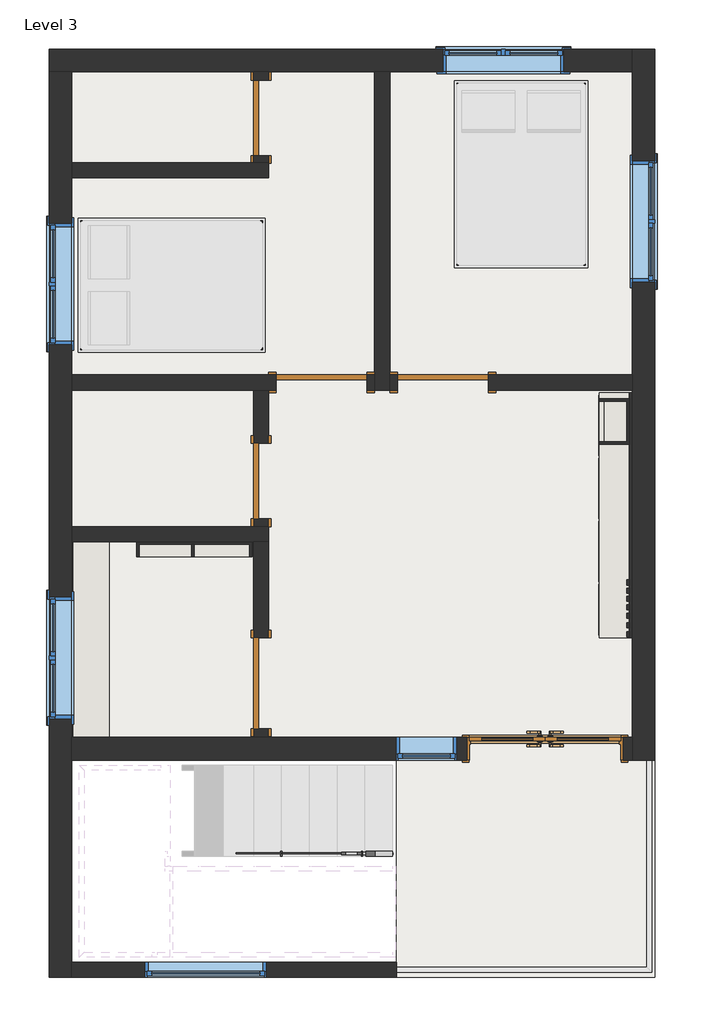
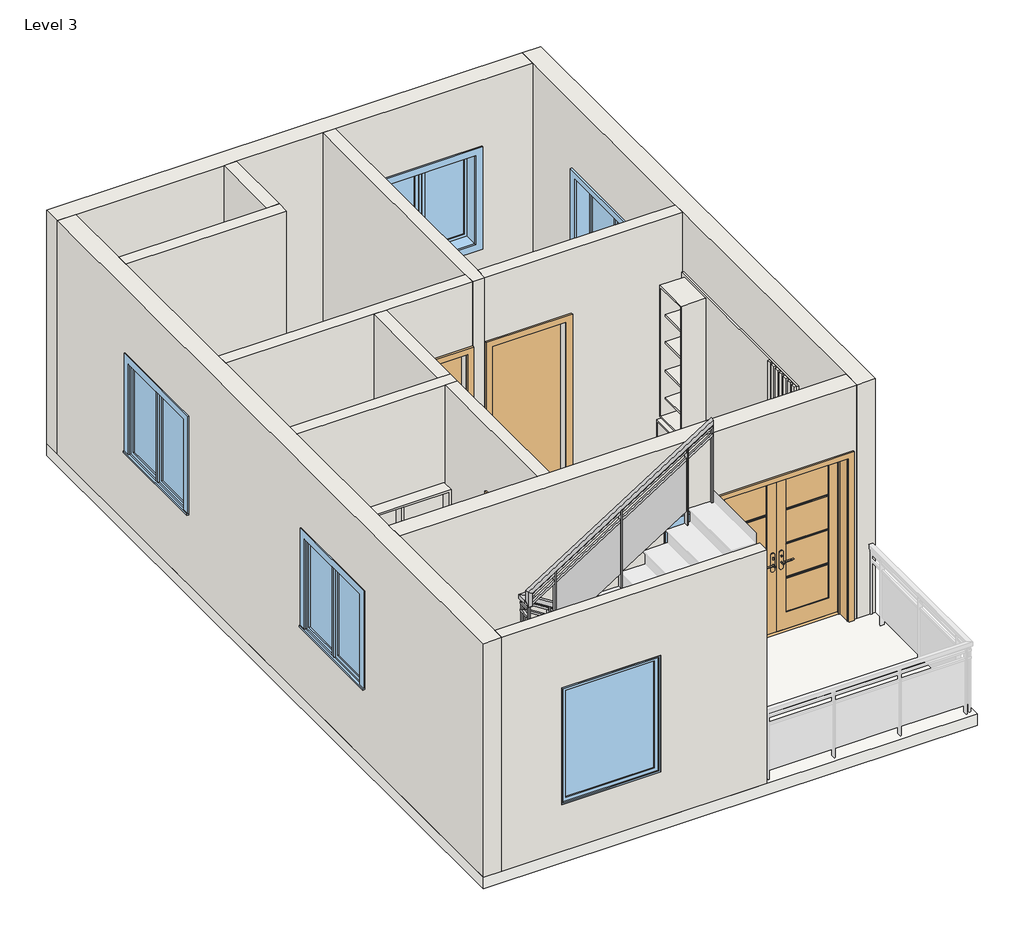
# One storey, part 1 of 2: 15 walls, 6 doors, 6 windows, 1 railing, 1 slab.
"""IFC4 building model written with IfcOpenShell, lengths in millimetres."""

from ifc_helpers import new_model, si_unit, frame, origin, place, context, project, spatial, polyline, outline, extrude, faceted_brep, transform, mapped, element, save
from components import m_door_exterior_double_full_glass_wood_clad_1524_x_2134mm_606f56d5, single_flush_2_5_e2b13fe9, door_686f89d2, door_16372e1c, walls_5_walls_1_1b2d60d9, walls_6_walls_2_a14d7d6d, window_534dcd48, window_fc882ab3, fixed_4_86eadd64

model = new_model("IFC4")

# Units and contexts
model_context = context("Model", 3, world=origin())
ifc_project = project(units=[si_unit("LENGTHUNIT", "METRE", prefix="MILLI")], contexts=[model_context])

# Site, building, storey
site = spatial("IfcSite", under=ifc_project)
building = spatial("IfcBuilding", under=site)
storey = spatial("IfcBuildingStorey", under=building, Name="Level 3", Elevation=6400.8)

# Doors
placement = place(None, origin())
m_door_exterior_double_full_glass_wood_clad_1524_x_2134mm_shape = m_door_exterior_double_full_glass_wood_clad_1524_x_2134mm_606f56d5(model_context)
element("IfcDoor", 1, ObjectType="M_Door-Exterior-Double-Full Glass-Wood_Clad : 1524 x 2134mm", at=placement, inside=storey, context=model_context, shape_type="MappedRepresentation", body=[
    mapped(m_door_exterior_double_full_glass_wood_clad_1524_x_2134mm_shape, transform((-1708.6112714, -4701.782676, 6400.8), x_axis=(1.0, 0.0, 0.0), y_axis=(0.0, 1.0, 0.0), z_axis=(0.0, 0.0, 1.0))),
])
single_flush_2_5_shape = single_flush_2_5_e2b13fe9(model_context)
element("IfcDoor", 2, ObjectType="Single-Flush : 2.5'", at=placement, inside=storey, context=model_context, shape_type="MappedRepresentation", body=[
    mapped(single_flush_2_5_shape, transform((-4566.1112714, -2012.557676, 6400.8), x_axis=(0.0, -1.0, 0.0), y_axis=(1.0, 0.0, 0.0), z_axis=(0.0, 0.0, 1.0))),
])
element("IfcDoor", 3, ObjectType="Single-Flush : 2.5'", at=placement, inside=storey, context=model_context, shape_type="MappedRepresentation", body=[
    mapped(single_flush_2_5_shape, transform((-4566.1112714, 1638.692324, 6400.8), x_axis=(0.0, -1.0, 0.0), y_axis=(1.0, 0.0, 0.0), z_axis=(0.0, 0.0, 1.0))),
])
door_shape = door_686f89d2(model_context)
element("IfcDoor", 4, ObjectType="Single-Flush : 36\" x 84\"", at=placement, inside=storey, context=model_context, shape_type="MappedRepresentation", body=[
    mapped(door_shape, transform((-4566.1112714, -4044.557676, 6400.8), x_axis=(0.0, -1.0, 0.0), y_axis=(1.0, 0.0, 0.0), z_axis=(0.0, 0.0, 1.0))),
])
element("IfcDoor", 5, ObjectType="Single-Flush : 36\" x 84\"", at=placement, inside=storey, context=model_context, shape_type="MappedRepresentation", body=[
    mapped(door_shape, transform((-2737.3112714, -1021.957676, 6400.8), x_axis=(-1.0, 0.0, 0.0), y_axis=(0.0, -1.0, 0.0), z_axis=(0.0, 0.0, 1.0))),
])
door_2_shape = door_16372e1c(model_context)
element("IfcDoor", 6, ObjectType="Single-Flush : 36\" x 84\"", at=placement, inside=storey, context=model_context, shape_type="MappedRepresentation", body=[
    mapped(door_2_shape, transform((-3956.5112714, -1021.957676, 6400.8), x_axis=(1.0, 0.0, 0.0), y_axis=(0.0, 1.0, 0.0), z_axis=(0.0, 0.0, 1.0))),
])

# Railing
element("IfcRailing", 7, ObjectType="Glass Panel - Bottom Fill", at=placement, inside=storey, context=model_context, shape_type="SolidModel", body=[
    faceted_brep([(-5531.3112714, -5886.057676, 9060.8727273), (-5480.5112714, -5886.057676, 9032.986276), (-5480.5112714, -5936.857676, 9032.986276), (-5531.3112714, -5936.857676, 9060.8727273), (-3245.3112714, -5886.057676, 10515.6), (-3245.3112714, -5936.857676, 10515.6), (-3245.3112714, -5936.857676, 10455.386276), (-3245.3112714, -5886.057676, 10455.386276)], [[[0, 1, 2, 3]], [[4, 5, 6, 7]], [[1, 0, 4, 7]], [[2, 1, 7, 6]], [[3, 2, 6, 5]], [[0, 3, 5, 4]]]),
    faceted_brep([(-5480.5112714, -5886.057676, 8915.4), (-5531.3112714, -5886.057676, 8915.4), (-5531.3112714, -5936.857676, 8864.6), (-5480.5112714, -5936.857676, 8864.6), (-5480.5112714, -5860.657676, 8864.6), (-5480.5112714, -5860.657676, 8915.4), (-5531.3112714, -5860.657676, 8864.6), (-5531.3112714, -5860.657676, 8915.4), (-3245.3112714, -5784.457676, 7493.0), (-3245.3112714, -5784.457676, 7432.786276), (-3245.3112714, -5733.657676, 7432.786276), (-3245.3112714, -5733.657676, 7493.0), (-5404.3112714, -5784.457676, 8866.9090909), (-5455.1112714, -5784.457676, 8839.0226396), (-5455.1112714, -5733.657676, 8839.0226396), (-5404.3112714, -5733.657676, 8866.9090909), (-5404.3112714, -5784.457676, 8915.4), (-5455.1112714, -5784.457676, 8864.6), (-5455.1112714, -5733.657676, 8864.6), (-5404.3112714, -5733.657676, 8915.4), (-5480.5112714, -5784.457676, 8915.4), (-5480.5112714, -5784.457676, 8864.6), (-5531.3112714, -5733.657676, 8864.6), (-5531.3112714, -5733.657676, 8915.4)], [[[0, 1, 2, 3]], [[4, 5, 0, 3]], [[6, 4, 3, 2]], [[7, 6, 2, 1]], [[5, 7, 1, 0]], [[8, 9, 10, 11]], [[9, 8, 12, 13]], [[10, 9, 13, 14]], [[11, 10, 14, 15]], [[8, 11, 15, 12]], [[13, 12, 16, 17]], [[14, 13, 17, 18]], [[15, 14, 18, 19]], [[12, 15, 19, 16]], [[17, 16, 20, 21]], [[18, 17, 21, 22]], [[19, 18, 22, 23]], [[16, 19, 23, 20]], [[21, 20, 5, 4]], [[22, 21, 4, 6]], [[23, 22, 6, 7]], [[20, 23, 7, 5]]]),
    faceted_brep([(-5480.5112714, -5886.057676, 8915.4), (-5480.5112714, -5936.857676, 8864.6), (-5531.3112714, -5936.857676, 8864.6), (-5531.3112714, -5886.057676, 8915.4), (-5480.5112714, -5886.057676, 9032.986276), (-5531.3112714, -5886.057676, 9060.8727273), (-5531.3112714, -5936.857676, 9060.8727273), (-5480.5112714, -5936.857676, 9032.986276)], [[[0, 1, 2, 3]], [[4, 5, 6, 7]], [[1, 0, 4, 7]], [[2, 1, 7, 6]], [[3, 2, 6, 5]], [[0, 3, 5, 4]]]),
    faceted_brep([(-3245.3112714, -5771.757676, 7406.453431), (-3245.3112714, -5771.757676, 7376.346569), (-3245.3112714, -5746.357676, 7376.346569), (-3245.3112714, -5746.357676, 7406.453431), (-5476.8130227, -5771.757676, 8826.5), (-5484.2095201, -5771.757676, 8801.1), (-5484.2095201, -5746.357676, 8801.1), (-5476.8130227, -5746.357676, 8826.5), (-5493.2112714, -5771.757676, 8826.5), (-5493.2112714, -5771.757676, 8801.1), (-5518.6112714, -5746.357676, 8801.1), (-5518.6112714, -5746.357676, 8826.5), (-5493.2112714, -5898.757676, 8826.5), (-5518.6112714, -5898.757676, 8826.5), (-5518.6112714, -5898.757676, 8801.1), (-5493.2112714, -5898.757676, 8801.1)], [[[0, 1, 2, 3]], [[1, 0, 4, 5]], [[2, 1, 5, 6]], [[3, 2, 6, 7]], [[0, 3, 7, 4]], [[5, 4, 8, 9]], [[6, 5, 9, 10]], [[7, 6, 10, 11]], [[4, 7, 11, 8]], [[12, 13, 14, 15]], [[9, 8, 12, 15]], [[10, 9, 15, 14]], [[11, 10, 14, 13]], [[8, 11, 13, 12]]]),
    faceted_brep([(-5518.6112714, -5898.757676, 8982.4079765), (-5518.6112714, -5898.757676, 8952.3011144), (-5518.6112714, -5924.157676, 8952.3011144), (-5518.6112714, -5924.157676, 8982.4079765), (-3245.3112714, -5898.757676, 10429.053431), (-3245.3112714, -5924.157676, 10429.053431), (-3245.3112714, -5924.157676, 10398.946569), (-3245.3112714, -5898.757676, 10398.946569)], [[[0, 1, 2, 3]], [[4, 5, 6, 7]], [[1, 0, 4, 7]], [[2, 1, 7, 6]], [[3, 2, 6, 5]], [[0, 3, 5, 4]]]),
    faceted_brep([(-3245.3112714, -5771.757676, 7304.853431), (-3245.3112714, -5771.757676, 7274.746569), (-3245.3112714, -5746.357676, 7274.746569), (-3245.3112714, -5746.357676, 7304.853431), (-5476.8130227, -5771.757676, 8724.9), (-5484.2095201, -5771.757676, 8699.5), (-5484.2095201, -5746.357676, 8699.5), (-5476.8130227, -5746.357676, 8724.9), (-5493.2112714, -5771.757676, 8724.9), (-5493.2112714, -5771.757676, 8699.5), (-5518.6112714, -5746.357676, 8699.5), (-5518.6112714, -5746.357676, 8724.9), (-5493.2112714, -5898.757676, 8724.9), (-5518.6112714, -5898.757676, 8724.9), (-5518.6112714, -5898.757676, 8699.5), (-5493.2112714, -5898.757676, 8699.5)], [[[0, 1, 2, 3]], [[1, 0, 4, 5]], [[2, 1, 5, 6]], [[3, 2, 6, 7]], [[0, 3, 7, 4]], [[5, 4, 8, 9]], [[6, 5, 9, 10]], [[7, 6, 10, 11]], [[4, 7, 11, 8]], [[12, 13, 14, 15]], [[9, 8, 12, 15]], [[10, 9, 15, 14]], [[11, 10, 14, 13]], [[8, 11, 13, 12]]]),
    faceted_brep([(-5518.6112714, -5898.757676, 8880.8079765), (-5518.6112714, -5898.757676, 8850.7011144), (-5518.6112714, -5924.157676, 8850.7011144), (-5518.6112714, -5924.157676, 8880.8079765), (-3245.3112714, -5898.757676, 10327.453431), (-3245.3112714, -5924.157676, 10327.453431), (-3245.3112714, -5924.157676, 10297.346569), (-3245.3112714, -5898.757676, 10297.346569)], [[[0, 1, 2, 3]], [[4, 5, 6, 7]], [[1, 0, 4, 7]], [[2, 1, 7, 6]], [[3, 2, 6, 5]], [[0, 3, 5, 4]]]),
    extrude(outline(polyline([(10249.2999123, -3569.1612714), (9245.6, -3569.1612714), (9245.6, -3556.4612714), (10257.3817305, -3556.4612714), (10249.2999123, -3569.1612714)])), frame((0.0, -5936.857676, 0.0), z_axis=(0.0, 1.0, 0.0), x_axis=(0.0, 0.0, 1.0)), (0.0, 0.0, 1.0), 50.8),
    extrude(outline(polyline([(8910.7818182, -4375.6112714), (9428.0181818, -3562.8112714), (10095.3011144, -3562.8112714), (9578.0647508, -4375.6112714), (8910.7818182, -4375.6112714)])), frame((0.0, -5917.992833, 0.0), z_axis=(0.0, 1.0, 0.0), x_axis=(0.0, 0.0, 1.0)), (0.0, 0.0, 1.0), 6.35),
    extrude(outline(polyline([(9732.0635487, -4381.9612714), (8712.2, -4381.9612714), (8712.2, -4369.2612714), (9740.1453669, -4369.2612714), (9732.0635487, -4381.9612714)])), frame((0.0, -5936.857676, 0.0), z_axis=(0.0, 1.0, 0.0), x_axis=(0.0, 0.0, 1.0)), (0.0, 0.0, 1.0), 50.8),
    extrude(outline(polyline([(8377.3818182, -5188.4112714), (8894.6181818, -4375.6112714), (9578.0647508, -4375.6112714), (9060.8283872, -5188.4112714), (8377.3818182, -5188.4112714)])), frame((0.0, -5917.992833, 0.0), z_axis=(0.0, 1.0, 0.0), x_axis=(0.0, 0.0, 1.0)), (0.0, 0.0, 1.0), 6.35),
    extrude(outline(polyline([(9214.8271851, -5194.7612714), (8356.6, -5194.7612714), (8356.6, -5182.0612714), (9222.9090032, -5182.0612714), (9214.8271851, -5194.7612714)])), frame((0.0, -5936.857676, 0.0), z_axis=(0.0, 1.0, 0.0), x_axis=(0.0, 0.0, 1.0)), (0.0, 0.0, 1.0), 50.8),
    extrude(outline(polyline([(8665.2635487, -5182.0612714), (7645.4, -5182.0612714), (7645.4, -5169.3612714), (8657.1817305, -5169.3612714), (8665.2635487, -5182.0612714)])), frame((0.0, -5784.457676, 0.0), z_axis=(0.0, 1.0, 0.0), x_axis=(0.0, 0.0, 1.0)), (0.0, 0.0, 1.0), 50.8),
    extrude(outline(polyline([(7310.5818182, -4362.9112714), (7985.946569, -4362.9112714), (8503.1829326, -5175.7112714), (7827.8181818, -5175.7112714), (7310.5818182, -4362.9112714)])), frame((0.0, -5758.872519, 0.0), z_axis=(0.0, 1.0, 0.0), x_axis=(0.0, 0.0, 1.0)), (0.0, 0.0, 1.0), 6.35),
    extrude(outline(polyline([(8148.0271851, -4369.2612714), (7289.8, -4369.2612714), (7289.8, -4356.5612714), (8139.9453669, -4356.5612714), (8148.0271851, -4369.2612714)])), frame((0.0, -5784.457676, 0.0), z_axis=(0.0, 1.0, 0.0), x_axis=(0.0, 0.0, 1.0)), (0.0, 0.0, 1.0), 50.8),
    extrude(outline(polyline([(6777.1818182, -3550.1112714), (7468.7102054, -3550.1112714), (7985.946569, -4362.9112714), (7294.4181818, -4362.9112714), (6777.1818182, -3550.1112714)])), frame((0.0, -5758.872519, 0.0), z_axis=(0.0, 1.0, 0.0), x_axis=(0.0, 0.0, 1.0)), (0.0, 0.0, 1.0), 6.35),
    extrude(outline(polyline([(7630.7908214, -3556.4612714), (6756.4, -3556.4612714), (6756.4, -3543.7612714), (7622.7090032, -3543.7612714), (7630.7908214, -3556.4612714)])), frame((0.0, -5784.457676, 0.0), z_axis=(0.0, 1.0, 0.0), x_axis=(0.0, 0.0, 1.0)), (0.0, 0.0, 1.0), 50.8),
    extrude(outline(polyline([(-5515.4362714, -5901.932676), (-5496.3862714, -5901.932676), (-5496.3862714, -5920.982676), (-5515.4362714, -5920.982676), (-5515.4362714, -5901.932676)])), frame((0.0, 0.0, 8001.0), z_axis=(0.0, 0.0, 1.0), x_axis=(1.0, 0.0, 0.0)), (0.0, 0.0, 1.0), 863.6),
    extrude(outline(polyline([(-5496.3862714, -5768.582676), (-5515.4362714, -5768.582676), (-5515.4362714, -5749.532676), (-5496.3862714, -5749.532676), (-5496.3862714, -5768.582676)])), frame((0.0, 0.0, 8001.0), z_axis=(0.0, 0.0, 1.0), x_axis=(1.0, 0.0, 0.0)), (0.0, 0.0, 1.0), 863.6),
    extrude(outline(polyline([(-5470.9862714, -5768.582676), (-5490.0362714, -5768.582676), (-5490.0362714, -5749.532676), (-5470.9862714, -5749.532676), (-5470.9862714, -5768.582676)])), frame((0.0, 0.0, 8001.0), z_axis=(0.0, 0.0, 1.0), x_axis=(1.0, 0.0, 0.0)), (0.0, 0.0, 1.0), 863.6),
    extrude(outline(polyline([(10447.3044578, -3258.0112714), (9423.4, -3258.0112714), (9423.4, -3238.9612714), (10459.4271851, -3238.9612714), (10447.3044578, -3258.0112714)])), frame((0.0, -5920.982676, 0.0), z_axis=(0.0, 1.0, 0.0), x_axis=(0.0, 0.0, 1.0)), (0.0, 0.0, 1.0), 19.05),
    extrude(outline(polyline([(7440.8680941, -3258.0112714), (6578.6, -3258.0112714), (6578.6, -3238.9612714), (7428.7453669, -3238.9612714), (7440.8680941, -3258.0112714)])), frame((0.0, -5768.582676, 0.0), z_axis=(0.0, 1.0, 0.0), x_axis=(0.0, 0.0, 1.0)), (0.0, 0.0, 1.0), 19.05),
])

# Slab
element("IfcSlab", 8, ObjectType="6\"", at=placement, inside=storey, context=model_context, shape_type="SweptSolid", body=[
    extrude(outline(polyline([(-603.7112714, 2330.842324), (-603.7112714, -7003.657676), (-6699.7112714, -7003.657676), (-6699.7112714, 2330.842324), (-603.7112714, 2330.842324)]), holes=[polyline([(-3209.2681702, -4819.257676), (-6473.1681702, -4819.257676), (-6473.1681702, -6851.257676), (-3209.2681702, -6851.257676), (-3209.2681702, -4819.257676)])]), frame((0.0, 0.0, 6248.4), z_axis=(0.0, 0.0, 1.0), x_axis=(1.0, 0.0, 0.0)), (0.0, 0.0, 1.0), 152.4),
])

# Walls
element("IfcWall", 9, ObjectType="6\"", at=placement, inside=storey, context=model_context, shape_type="Brep", body=[
    faceted_brep([(-3423.1112714, 2102.242324, 6400.8), (-3423.1112714, -945.757676, 6400.8), (-3423.1112714, -1098.157676, 6400.8), (-3423.1112714, -1098.157676, 9448.8), (-3423.1112714, -945.757676, 9448.8), (-3423.1112714, 2102.242324, 9448.8), (-3270.7112714, 2102.242324, 6400.8), (-3270.7112714, 2102.242324, 9448.8), (-3270.7112714, -945.757676, 9448.8), (-3270.7112714, -1098.157676, 9448.8), (-3270.7112714, -1098.157676, 6400.8), (-3270.7112714, -945.757676, 6400.8)], [[[0, 1, 2, 3, 4, 5]], [[6, 7, 8, 9, 10, 11]], [[2, 1, 0, 6, 11, 10]], [[5, 4, 3, 9, 8, 7]], [[0, 5, 7, 6]], [[3, 2, 10, 9]]]),
])
element("IfcWall", 10, ObjectType="6\"", at=placement, inside=storey, context=model_context, shape_type="Brep", body=[
    faceted_brep([(-3423.1112714, -945.757676, 6400.8), (-3499.3112714, -945.757676, 6400.8), (-3499.3112714, -945.757676, 8534.4), (-4413.7112714, -945.757676, 8534.4), (-4413.7112714, -945.757676, 6400.8), (-6471.1112714, -945.757676, 6400.8), (-6471.1112714, -945.757676, 9448.8), (-3423.1112714, -945.757676, 9448.8), (-3499.3112714, -1098.157676, 8534.4), (-3499.3112714, -1098.157676, 6400.8), (-3423.1112714, -1098.157676, 6400.8), (-3423.1112714, -1098.157676, 9448.8), (-4489.9112714, -1098.157676, 9448.8), (-4642.3112714, -1098.157676, 9448.8), (-6471.1112714, -1098.157676, 9448.8), (-6471.1112714, -1098.157676, 6400.8), (-4642.3112714, -1098.157676, 6400.8), (-4489.9112714, -1098.157676, 6400.8), (-4413.7112714, -1098.157676, 6400.8), (-4413.7112714, -1098.157676, 8534.4)], [[[0, 1, 2, 3, 4, 5, 6, 7]], [[8, 9, 10, 11, 12, 13, 14, 15, 16, 17, 18, 19]], [[10, 9, 1, 0]], [[18, 17, 16, 15, 5, 4]], [[7, 6, 14, 13, 12, 11]], [[6, 5, 15, 14]], [[0, 7, 11, 10]], [[2, 1, 9, 8]], [[3, 2, 8, 19]], [[4, 3, 19, 18]]]),
])
element("IfcWall", 11, ObjectType="6\"", at=placement, inside=storey, context=model_context, shape_type="SweptSolid", body=[
    extrude(outline(polyline([(6400.8, -3270.7112714), (6400.8, -3194.5112714), (8534.4, -3194.5112714), (8534.4, -2280.1112714), (6400.8, -2280.1112714), (6400.8, -832.3112714), (9448.8, -832.3112714), (9448.8, -3270.7112714), (6400.8, -3270.7112714)])), frame((0.0, -1098.157676, 0.0), z_axis=(0.0, 1.0, 0.0), x_axis=(0.0, 0.0, 1.0)), (0.0, 0.0, 1.0), 152.4),
])
element("IfcWall", 12, ObjectType="6\"", at=placement, inside=storey, context=model_context, shape_type="Brep", body=[
    faceted_brep([(-6471.1112714, -2622.157676, 6400.8), (-4642.3112714, -2622.157676, 6400.8), (-4489.9112714, -2622.157676, 6400.8), (-4489.9112714, -2622.157676, 9448.8), (-4642.3112714, -2622.157676, 9448.8), (-6471.1112714, -2622.157676, 9448.8), (-6471.1112714, -2469.757676, 6400.8), (-6471.1112714, -2469.757676, 9448.8), (-4642.3112714, -2469.757676, 9448.8), (-4489.9112714, -2469.757676, 9448.8), (-4489.9112714, -2469.757676, 6400.8), (-4642.3112714, -2469.757676, 6400.8)], [[[0, 1, 2, 3, 4, 5]], [[6, 7, 8, 9, 10, 11]], [[2, 1, 0, 6, 11, 10]], [[5, 4, 3, 9, 8, 7]], [[0, 5, 7, 6]], [[3, 2, 10, 9]]]),
])
element("IfcWall", 13, ObjectType="6\"", at=placement, inside=storey, context=model_context, shape_type="SweptSolid", body=[
    extrude(outline(polyline([(-2393.557676, 8534.4), (-2393.557676, 6400.8), (-2469.757676, 6400.8), (-2469.757676, 9448.8), (-1098.157676, 9448.8), (-1098.157676, 6400.8), (-1631.557676, 6400.8), (-1631.557676, 8534.4), (-2393.557676, 8534.4)])), frame((-4642.3112714, 0.0, 0.0), z_axis=(1.0, 0.0, 0.0), x_axis=(0.0, 1.0, 0.0)), (0.0, 0.0, 1.0), 152.4),
])
element("IfcWall", 14, ObjectType="6\"", at=placement, inside=storey, context=model_context, shape_type="SweptSolid", body=[
    extrude(outline(polyline([(-4501.757676, 8534.4), (-4501.757676, 6400.8), (-4590.657676, 6400.8), (-4590.657676, 9448.8), (-2622.157676, 9448.8), (-2622.157676, 6400.8), (-3587.357676, 6400.8), (-3587.357676, 8534.4), (-4501.757676, 8534.4)])), frame((-4642.3112714, 0.0, 0.0), z_axis=(1.0, 0.0, 0.0), x_axis=(0.0, 1.0, 0.0)), (0.0, 0.0, 1.0), 152.4),
])
element("IfcWall", 15, ObjectType="6\"", at=placement, inside=storey, context=model_context, shape_type="SweptSolid", body=[
    extrude(outline(polyline([(1257.692324, 8534.4), (1257.692324, 6400.8), (1187.842324, 6400.8), (1187.842324, 9448.8), (2102.242324, 9448.8), (2102.242324, 6400.8), (2019.692324, 6400.8), (2019.692324, 8534.4), (1257.692324, 8534.4)])), frame((-4642.3112714, 0.0, 0.0), z_axis=(1.0, 0.0, 0.0), x_axis=(0.0, 1.0, 0.0)), (0.0, 0.0, 1.0), 152.4),
])
element("IfcWall", 16, ObjectType="6\"", at=placement, inside=storey, context=model_context, shape_type="Brep", body=[
    faceted_brep([(-4489.9112714, 1187.842324, 6400.8), (-4642.3112714, 1187.842324, 6400.8), (-6471.1112714, 1187.842324, 6400.8), (-6471.1112714, 1187.842324, 9448.8), (-4642.3112714, 1187.842324, 9448.8), (-4489.9112714, 1187.842324, 9448.8), (-4489.9112714, 1035.442324, 6400.8), (-4489.9112714, 1035.442324, 9448.8), (-6471.1112714, 1035.442324, 9448.8), (-6471.1112714, 1035.442324, 6400.8)], [[[0, 1, 2, 3, 4, 5]], [[6, 7, 8, 9]], [[2, 1, 0, 6, 9]], [[5, 4, 3, 8, 7]], [[3, 2, 9, 8]], [[0, 5, 7, 6]]]),
])
element("IfcWall", 17, ObjectType="6\"", at=placement, inside=storey, context=model_context, shape_type="SweptSolid", body=[
    extrude(outline(polyline([(6400.8, -3204.6473712), (9448.8, -3204.6473712), (9448.8, -6471.1112714), (6400.8, -6471.1112714), (6400.8, -3204.6473712)]), holes=[polyline([(8534.4, -5733.2293213), (8534.4, -4514.0293213), (7010.4, -4514.0293213), (7010.4, -5733.2293213), (8534.4, -5733.2293213)])]), frame((0.0, -7003.657676, 0.0), z_axis=(0.0, 1.0, 0.0), x_axis=(0.0, 0.0, 1.0)), (0.0, 0.0, 1.0), 152.4),
])
element("IfcWall", 18, ObjectType="9\"", at=placement, inside=storey, context=model_context, shape_type="Brep", body=[
    faceted_brep([(-6699.7112714, 2102.242324, 6400.8), (-6471.1112714, 2102.242324, 6400.8), (-4642.3112714, 2102.242324, 6400.8), (-4489.9112714, 2102.242324, 6400.8), (-3423.1112714, 2102.242324, 6400.8), (-3270.7112714, 2102.242324, 6400.8), (-832.3112714, 2102.242324, 6400.8), (-832.3112714, 2102.242324, 9448.8), (-3270.7112714, 2102.242324, 9448.8), (-3423.1112714, 2102.242324, 9448.8), (-4489.9112714, 2102.242324, 9448.8), (-4642.3112714, 2102.242324, 9448.8), (-6471.1112714, 2102.242324, 9448.8), (-6699.7112714, 2102.242324, 9448.8), (-1518.1112714, 2102.242324, 8534.4), (-1518.1112714, 2102.242324, 7315.2), (-2737.3112714, 2102.242324, 7315.2), (-2737.3112714, 2102.242324, 8534.4), (-6699.7112714, 2330.842324, 6400.8), (-6699.7112714, 2330.842324, 9448.8), (-832.3112714, 2330.842324, 9448.8), (-832.3112714, 2330.842324, 6400.8), (-1518.1112714, 2330.842324, 8534.4), (-2737.3112714, 2330.842324, 8534.4), (-2737.3112714, 2330.842324, 7315.2), (-1518.1112714, 2330.842324, 7315.2)], [[[0, 1, 2, 3, 4, 5, 6, 7, 8, 9, 10, 11, 12, 13], [14, 15, 16, 17]], [[18, 19, 20, 21], [22, 23, 24, 25]], [[6, 5, 4, 3, 2, 1, 0, 18, 21]], [[13, 12, 11, 10, 9, 8, 7, 20, 19]], [[0, 13, 19, 18]], [[7, 6, 21, 20]], [[15, 14, 22, 25]], [[16, 15, 25, 24]], [[17, 16, 24, 23]], [[14, 17, 23, 22]]]),
])
element("IfcWall", 19, ObjectType="9\"", at=placement, inside=storey, context=model_context, shape_type="Brep", body=[
    faceted_brep([(-6471.1112714, -7003.657676, 6400.8), (-6471.1112714, -6851.257676, 6400.8), (-6471.1112714, -4819.257676, 6400.8), (-6471.1112714, -4590.657676, 6400.8), (-6471.1112714, -2622.157676, 6400.8), (-6471.1112714, -2469.757676, 6400.8), (-6471.1112714, -1098.157676, 6400.8), (-6471.1112714, -945.757676, 6400.8), (-6471.1112714, 1035.442324, 6400.8), (-6471.1112714, 1187.842324, 6400.8), (-6471.1112714, 2102.242324, 6400.8), (-6471.1112714, 2102.242324, 9448.8), (-6471.1112714, 1187.842324, 9448.8), (-6471.1112714, 1035.442324, 9448.8), (-6471.1112714, -945.757676, 9448.8), (-6471.1112714, -1098.157676, 9448.8), (-6471.1112714, -2469.757676, 9448.8), (-6471.1112714, -2622.157676, 9448.8), (-6471.1112714, -4590.657676, 9448.8), (-6471.1112714, -4819.257676, 9448.8), (-6471.1112714, -6851.257676, 9448.8), (-6471.1112714, -7003.657676, 9448.8), (-6471.1112714, -3180.957676, 8534.4), (-6471.1112714, -3180.957676, 7315.2), (-6471.1112714, -4400.157676, 7315.2), (-6471.1112714, -4400.157676, 8534.4), (-6471.1112714, 578.242324, 8534.4), (-6471.1112714, 578.242324, 7315.2), (-6471.1112714, -640.957676, 7315.2), (-6471.1112714, -640.957676, 8534.4), (-6699.7112714, -7003.657676, 6400.8), (-6699.7112714, -7003.657676, 9448.8), (-6699.7112714, 2102.242324, 9448.8), (-6699.7112714, 2102.242324, 6400.8), (-6699.7112714, -3180.957676, 8534.4), (-6699.7112714, -4400.157676, 8534.4), (-6699.7112714, -4400.157676, 7315.2), (-6699.7112714, -3180.957676, 7315.2), (-6699.7112714, 578.242324, 8534.4), (-6699.7112714, -640.957676, 8534.4), (-6699.7112714, -640.957676, 7315.2), (-6699.7112714, 578.242324, 7315.2)], [[[0, 1, 2, 3, 4, 5, 6, 7, 8, 9, 10, 11, 12, 13, 14, 15, 16, 17, 18, 19, 20, 21], [22, 23, 24, 25], [26, 27, 28, 29]], [[30, 31, 32, 33], [34, 35, 36, 37], [38, 39, 40, 41]], [[10, 9, 8, 7, 6, 5, 4, 3, 2, 1, 0, 30, 33]], [[21, 20, 19, 18, 17, 16, 15, 14, 13, 12, 11, 32, 31]], [[0, 21, 31, 30]], [[11, 10, 33, 32]], [[23, 22, 34, 37]], [[24, 23, 37, 36]], [[25, 24, 36, 35]], [[22, 25, 35, 34]], [[27, 26, 38, 41]], [[28, 27, 41, 40]], [[29, 28, 40, 39]], [[26, 29, 39, 38]]]),
])
element("IfcWall", 20, ObjectType="9\"", at=placement, inside=storey, context=model_context, shape_type="Brep", body=[
    faceted_brep([(-832.3112714, 2330.842324, 6400.8), (-832.3112714, 2102.242324, 6400.8), (-832.3112714, -945.757676, 6400.8), (-832.3112714, -1098.157676, 6400.8), (-832.3112714, -4590.657676, 6400.8), (-832.3112714, -4819.257676, 6400.8), (-832.3112714, -4819.257676, 9448.8), (-832.3112714, -4590.657676, 9448.8), (-832.3112714, -1098.157676, 9448.8), (-832.3112714, -945.757676, 9448.8), (-832.3112714, 2102.242324, 9448.8), (-832.3112714, 2330.842324, 9448.8), (-832.3112714, -12.307676, 8534.4), (-832.3112714, -12.307676, 7315.2), (-832.3112714, 1206.892324, 7315.2), (-832.3112714, 1206.892324, 8534.4), (-603.7112714, 2330.842324, 6400.8), (-603.7112714, 2330.842324, 9448.8), (-603.7112714, -4819.257676, 9448.8), (-603.7112714, -4819.257676, 6400.8), (-603.7112714, -12.307676, 8534.4), (-603.7112714, 1206.892324, 8534.4), (-603.7112714, 1206.892324, 7315.2), (-603.7112714, -12.307676, 7315.2)], [[[0, 1, 2, 3, 4, 5, 6, 7, 8, 9, 10, 11], [12, 13, 14, 15]], [[16, 17, 18, 19], [20, 21, 22, 23]], [[5, 4, 3, 2, 1, 0, 16, 19]], [[6, 5, 19, 18]], [[11, 10, 9, 8, 7, 6, 18, 17]], [[0, 11, 17, 16]], [[13, 12, 20, 23]], [[14, 13, 23, 22]], [[15, 14, 22, 21]], [[12, 15, 21, 20]]]),
])
element("IfcWall", 21, ObjectType="9\"", at=placement, inside=storey, context=model_context, shape_type="Brep", body=[
    faceted_brep([(-832.3112714, -4819.257676, 9448.8), (-6471.1112714, -4819.257676, 9448.8), (-6471.1112714, -4819.257676, 6400.8), (-2495.6112714, -4819.257676, 6400.8), (-2495.6112714, -4819.257676, 8559.4), (-921.6112714, -4819.257676, 8559.4), (-921.6112714, -4819.257676, 6400.8), (-832.3112714, -4819.257676, 6400.8), (-3207.2112714, -4819.257676, 8534.4), (-2597.6112714, -4819.257676, 8534.4), (-2597.6112714, -4819.257676, 6705.6), (-3207.2112714, -4819.257676, 6705.6), (-6471.1112714, -4590.657676, 9448.8), (-4642.3112714, -4590.657676, 9448.8), (-4489.9112714, -4590.657676, 9448.8), (-832.3112714, -4590.657676, 9448.8), (-832.3112714, -4590.657676, 6400.8), (-921.6112714, -4590.657676, 6400.8), (-921.6112714, -4590.657676, 8559.4), (-2495.6112714, -4590.657676, 8559.4), (-2495.6112714, -4590.657676, 6400.8), (-4489.9112714, -4590.657676, 6400.8), (-4642.3112714, -4590.657676, 6400.8), (-6471.1112714, -4590.657676, 6400.8), (-3207.2112714, -4590.657676, 8534.4), (-3207.2112714, -4590.657676, 6705.6), (-2597.6112714, -4590.657676, 6705.6), (-2597.6112714, -4590.657676, 8534.4)], [[[0, 1, 2, 3, 4, 5, 6, 7], [8, 9, 10, 11]], [[12, 13, 14, 15, 16, 17, 18, 19, 20, 21, 22, 23], [24, 25, 26, 27]], [[2, 23, 22, 21, 20, 3]], [[16, 7, 6, 17]], [[1, 0, 15, 14, 13, 12]], [[2, 1, 12, 23]], [[0, 7, 16, 15]], [[5, 18, 17, 6]], [[18, 5, 4, 19]], [[19, 4, 3, 20]], [[25, 24, 8, 11]], [[26, 25, 11, 10]], [[27, 26, 10, 9]], [[24, 27, 9, 8]]]),
])
walls_5_walls_1_shape = walls_5_walls_1_1b2d60d9(model_context)
element("IfcWall", 22, ObjectType="Walls 5 : Walls 1", at=placement, inside=storey, context=model_context, shape_type="MappedRepresentation", body=[
    mapped(walls_5_walls_1_shape, transform((0.0, 0.0, 0.0), x_axis=(1.0, 0.0, 0.0), y_axis=(0.0, 1.0, 0.0), z_axis=(0.0, 0.0, 1.0))),
])
walls_6_walls_2_shape = walls_6_walls_2_a14d7d6d(model_context)
element("IfcWall", 23, ObjectType="Walls 6 : Walls 2", at=placement, inside=storey, context=model_context, shape_type="MappedRepresentation", body=[
    mapped(walls_6_walls_2_shape, transform((0.0, 0.0, 0.0), x_axis=(1.0, 0.0, 0.0), y_axis=(0.0, 1.0, 0.0), z_axis=(0.0, 0.0, 1.0))),
])

# Windows
window_shape = window_534dcd48(model_context)
element("IfcWindow", 24, ObjectType="Casement Dbl with Trim : 48\" x 48\"", at=placement, inside=storey, context=model_context, shape_type="MappedRepresentation", body=[
    mapped(window_shape, transform((-6566.3612714, -3790.557676, 6400.8), x_axis=(0.0, 1.0, 0.0), y_axis=(-1.0, 0.0, 0.0), z_axis=(0.0, 0.0, 1.0))),
])
element("IfcWindow", 25, ObjectType="Casement Dbl with Trim : 48\" x 48\"", at=placement, inside=storey, context=model_context, shape_type="MappedRepresentation", body=[
    mapped(window_shape, transform((-737.0612714, 597.292324, 6400.8), x_axis=(0.0, -1.0, 0.0), y_axis=(1.0, 0.0, 0.0), z_axis=(0.0, 0.0, 1.0))),
])
element("IfcWindow", 26, ObjectType="Casement Dbl with Trim : 48\" x 48\"", at=placement, inside=storey, context=model_context, shape_type="MappedRepresentation", body=[
    mapped(window_shape, transform((-2127.7112714, 2197.492324, 6400.8), x_axis=(1.0, 0.0, 0.0), y_axis=(0.0, 1.0, 0.0), z_axis=(0.0, 0.0, 1.0))),
])
element("IfcWindow", 27, ObjectType="Casement Dbl with Trim : 48\" x 48\"", at=placement, inside=storey, context=model_context, shape_type="MappedRepresentation", body=[
    mapped(window_shape, transform((-6566.3612714, -31.357676, 6400.8), x_axis=(0.0, 1.0, 0.0), y_axis=(-1.0, 0.0, 0.0), z_axis=(0.0, 0.0, 1.0))),
])
window_2_shape = window_fc882ab3(model_context)
element("IfcWindow", 28, ObjectType="Fixed : 24\" x 72\"", at=placement, inside=storey, context=model_context, shape_type="MappedRepresentation", body=[
    mapped(window_2_shape, transform((-2940.5112714, -4704.957676, 6400.8), x_axis=(-1.0, 0.0, 0.0), y_axis=(0.0, -1.0, 0.0), z_axis=(0.0, 0.0, 1.0))),
])
fixed_4_shape = fixed_4_86eadd64(model_context)
element("IfcWindow", 29, ObjectType="Fixed : 4'", at=placement, inside=storey, context=model_context, shape_type="MappedRepresentation", body=[
    mapped(fixed_4_shape, transform((-5161.7293213, -6927.457676, 6400.8), x_axis=(-1.0, 0.0, 0.0), y_axis=(0.0, -1.0, 0.0), z_axis=(0.0, 0.0, 1.0))),
])

save(model, "model.ifc")

# Revit data of these elements
# Type "M_Door-Exterior-Double-Full Glass-Wood_Clad : 1524 x 2134mm"
#   Type Mark = "9"
#   Assembly Code = "B2030100"
#   Analytic Construction = "French door, wood frame with double glass"
#   Top Rail = 0' - 4.72441"
#   Threshold Offset [instance default] = 0' - 0.59055"
#   Thickness = 0' - 1.37795"
#   Thermal Resistance (R) = 1.9158 (h·ft²·°F)/BTU
#   Swing Angle [instance default] = 90.00°
#   Stiles = 0' - 4.72441"
#   Rough Width = 5' - 1.9685"
#   Rough Height = 7' - 0.98425"
#   Panel Width = 2' - 6"
#   Door Offset [instance default] = 0' - 0"
#   Height = 7' - 0"
#   Width = 5' - 0"
#   Heat Transfer Coefficient (U) = 0.5220 BTU/(h·ft²·°F)
#   Bottom Rail = 0' - 9.05512"
#   Exterior Trim [instance default] = yes
#   Threshold [instance default] = yes
#   Show Grill [instance default] = yes
#   Function = 1
#   Trim Material = Cherry
#   Threshold Material = Cherry
#   Panel Material = Cherry
#   Glazing = Glass
#   Frame Material = Cherry
#   Door Handle Material = Aluminum
#   Visual Light Transmittance = 0
#   Solar Heat Gain Coefficient = 0
#   Wall Closure = (empty or 0)
#   Construction Type = (empty or 0)
# Type "Single-Flush : 2.5'"
#   Type Mark = "8"
#   Construction Type Id = "MDOOR"
#   Assembly Code = "C1020"
#   Analytic Construction = "Metal"
#   Thickness = 0' - 2"
#   Heat Transfer Coefficient (U) = 0.651978 BTU/(h·ft²·°F)
#   Height = 7' - 0"
#   Trim Projection Ext = 0' - 1"
#   Trim Projection Int = 0' - 1"
#   Trim Width = 0' - 3"
#   Width = 2' - 6"
#   Define Thermal Properties by = 1
#   Door Material = Door - Panel
#   Frame Material = Door - Frame
#   Visual Light Transmittance = 0
#   Solar Heat Gain Coefficient = 0
#   Function = (empty or 0)
#   Wall Closure = (empty or 0)
# Type "Single-Flush : 36\" x 84\""
#   Type Mark = "1"
#   Construction Type Id = "MDOOR"
#   Assembly Code = "C1020"
#   Analytic Construction = "Metal"
#   Thickness = 0' - 2"
#   Heat Transfer Coefficient (U) = 0.651978 BTU/(h·ft²·°F)
#   Height = 7' - 0"
#   Trim Projection Ext = 0' - 1"
#   Trim Projection Int = 0' - 1"
#   Trim Width = 0' - 3"
#   Width = 3' - 0"
#   Define Thermal Properties by = 1
#   Door Material = Door - Panel
#   Frame Material = Door - Frame
#   Visual Light Transmittance = 0
#   Solar Heat Gain Coefficient = 0
#   Function = (empty or 0)
#   Wall Closure = (empty or 0)
# Type "Glass Panel - Bottom Fill"
#   Assembly Code = "C2010400"
#   built-in parameter 1008612 = 0.0416667 (stored number, unit not read)
#   built-in parameter 1008611 = 0.0416667 (stored number, unit not read)
#   built-in parameter 1008609 = 0.333333 (stored number, unit not read)
#   built-in parameter 1008604 = 0.166667 (stored number, unit not read)
#   built-in parameter 1008603 = 0.166667 (stored number, unit not read)
#   Railing Height = 3' - 0"
#   built-in parameter 1008630 = 2
#   built-in parameter 1008610 = 2
#   built-in parameter 1008618 = Baluster - Square : 3/4"
# Type "6\""
#   Assembly Code = "B1010"
#   Function = 0
#   Layers, outside or top first: 0' - 6" "floor" (function 1)
# Type "6\""
#   Assembly Code = "B2010"
#   Layers, outside or top first: 0' - 6" "ext wall" (function 1)
# Type "9\""
#   Assembly Code = "B2010"
#   Layers, outside or top first: 0' - 9" "int wall" (function 1)
# Type "Casement Dbl with Trim : 48\" x 48\""
#   Type Mark = "10"
#   Construction Type Id = "GSP4R"
#   Assembly Code = "B2020100"
#   Analytic Construction = "1/8 in Pilkington single glazing"
#   Visual Light Transmittance = 0.9
#   Solar Heat Gain Coefficient = 0.78
#   Heat Transfer Coefficient (U) = 0.6496 BTU/(h·ft²·°F)
#   Height = 4' - 0"
#   Default Sill Height = 3' - 0"
#   Trim Projection - Ext. = 0' - 0 1/2"
#   Trim Projection - Int. = 0' - 0 3/4"
#   Trim Width - Exterior = 0' - 3 1/2"
#   Trim Width - Interior = 0' - 3 1/2"
#   Width = 4' - 0"
#   Window Inset = 0' - 0 3/4"
#   Define Thermal Properties by = 1
#   Glass Pane Material = Glass
#   Sash Material = Sash
#   Trim Exterior Material = Trim
#   Trim Interior Material = Trim
#   Wall Closure = (empty or 0)
# Type "Fixed : 24\" x 72\""
#   Type Mark = "7"
#   Construction Type Id = "GSP4R"
#   Assembly Code = "B2020100"
#   Analytic Construction = "1/8 in Pilkington single glazing"
#   Visual Light Transmittance = 0.9
#   Solar Heat Gain Coefficient = 0.78
#   Heat Transfer Coefficient (U) = 0.6496 BTU/(h·ft²·°F)
#   Height = 6' - 0"
#   Default Sill Height = 1' - 0"
#   Width = 2' - 0"
#   Window Inset = 0' - 0 3/4"
#   Define Thermal Properties by = 1
#   Glass Pane Material = Glass
#   Sash Material = Sash
#   Wall Closure = (empty or 0)
# Type "Fixed : 4'"
#   Type Mark = "13"
#   Construction Type Id = "GSP4R"
#   Assembly Code = "B2020100"
#   Analytic Construction = "1/8 in Pilkington single glazing"
#   Visual Light Transmittance = 0.9
#   Solar Heat Gain Coefficient = 0.78
#   Heat Transfer Coefficient (U) = 0.6496 BTU/(h·ft²·°F)
#   Height = 5' - 0"
#   Default Sill Height = 2' - 0"
#   Width = 4' - 0"
#   Window Inset = 0' - 0 3/4"
#   Define Thermal Properties by = 1
#   Glass Pane Material = Glass
#   Sash Material = Sash
#   Wall Closure = (empty or 0)
# Element 1 (IfcDoor, "M_Door-Exterior-Double-Full Glass-Wood_Clad : 1524 x 2134mm")
#   Threshold Offset = 0' - 0.59055"
#   Swing Angle = 90.00°
#   Door Offset = 0' - 0"
#   Threshold = yes
#   Show Grill = yes
#   Exterior Trim = yes
#   Phase Created = New Construction
#   Materials on its faces: "Cherry", "Aluminum", "Glass"
# Elements 2, 3 (IfcDoor, "Single-Flush : 2.5'")
#   Phase Created = New Construction
#   Materials on its faces: "Door - Frame", "Door - Panel"
# Elements 4, 5, 6 (IfcDoor, "Single-Flush : 36\" x 84\"")
#   Phase Created = New Construction
#   Materials on its faces: "Door - Frame", "Door - Panel"
# Element 7 (IfcRailing, "Glass Panel - Bottom Fill")
#   Phase Created = New Construction
#   Materials on its faces: "Glass"
# Element 8 (IfcSlab, "6\"")
#   Height Offset From Level = 0' - 0"
#   Phase Created = New Construction
#   Materials on its faces: "floor"
# Elements 9, 10, 11, 12, 13, 14, 15, 16, 17 (IfcWall, "6\"")
#   Top Offset = 0' - 0"
#   Base Offset = 0' - 0"
#   Unconnected Height = 10' - 0"
#   wall height = 10' - 0"
#   Phase Created = New Construction
#   Base Constraint = Level 3
#   Materials on its faces: "ext wall"
# Elements 18, 20, 21 (IfcWall, "9\"")
#   Top Offset = 0' - 0"
#   Base Offset = 0' - 0"
#   Unconnected Height = 10' - 0"
#   wall height = 10' - 0"
#   Phase Created = New Construction
#   Base Constraint = Level 3
#   Materials on its faces: "int wall"
# Element 19 (IfcWall, "9\"")
#   Top Offset = 0' - 0"
#   Base Offset = 0' - 0"
#   Unconnected Height = 10' - 0"
#   wall height = 10' - 0"
#   Phase Created = New Construction
#   Base Constraint = Level 3
#   Materials on its faces: "int wall", "ext wall"
# Element 22 (IfcWall, "Walls 5 : Walls 1")
#   Phase Created = New Construction
#   Materials on its faces: "drawers", "wood", "clear glass", "stone", "Default Wall"
# Element 23 (IfcWall, "Walls 6 : Walls 2")
#   Phase Created = New Construction
#   Materials on its faces: "drawers", "metal", "wood"
# Element 24 (IfcWindow, "Casement Dbl with Trim : 48\" x 48\"")
#   Mark = "11"
#   Phase Created = New Construction
#   Materials on its faces: "Sash", "Trim", "Glass"
# Element 25 (IfcWindow, "Casement Dbl with Trim : 48\" x 48\"")
#   Mark = "12"
#   Phase Created = New Construction
#   Materials on its faces: "Sash", "Trim", "Glass"
# Element 26 (IfcWindow, "Casement Dbl with Trim : 48\" x 48\"")
#   Mark = "13"
#   Phase Created = New Construction
#   Materials on its faces: "Sash", "Trim", "Glass"
# Element 27 (IfcWindow, "Casement Dbl with Trim : 48\" x 48\"")
#   Mark = "21"
#   Phase Created = New Construction
#   Materials on its faces: "Sash", "Trim", "Glass"
# Element 28 (IfcWindow, "Fixed : 24\" x 72\"")
#   Mark = "14"
#   Phase Created = New Construction
#   Materials on its faces: "Sash", "Glass"
# Element 29 (IfcWindow, "Fixed : 4'")
#   Mark = "19"
#   Phase Created = New Construction
#   Materials on its faces: "Sash", "Glass"
# Materials
#   "Cherry": class "Wood", colour RGB 226 177 128, transparency 0, Description = "Prunus Serotina", Cost = 0
#   "Glass": class "Glass", colour RGB 0 128 192, transparency 0.75, Description = "Soda Lime Glass", Cost = 0
#   "Aluminum": class "Metal", colour RGB 247 247 247, transparency 0, Description = "Aluminum 6061", Cost = 0
#   "Door - Panel": class "Wood", colour RGB 210 159 95, transparency 0
#   "Door - Frame": colour RGB 118 70 51, transparency 0
#   "floor": class "Generic", colour RGB 138 129 123, transparency 0, Cost = 0
#   "ext wall": class "Generic", colour RGB 219 210 180, transparency 0, Cost = 0
#   "int wall": class "Generic", colour RGB 230 213 172, transparency 0, Cost = 0
#   "Sash": class "Wood", colour RGB 224 178 126, transparency 0
#   "Trim": class "Wood", colour RGB 224 178 126, transparency 0
#   "drawers": class "Generic", colour RGB 121 66 39, transparency 0, Cost = 0
#   "wood": class "Generic", colour RGB 255 226 181, transparency 0, Cost = 0
#   "clear glass": class "Generic", colour RGB 141 181 235, transparency 0.9, Cost = 0
#   "stone": class "Generic", colour RGB 125 126 130, transparency 0, Cost = 0
#   "Default Wall": colour RGB 128 128 128, transparency 0
#   "metal": class "Generic", colour RGB 76 25 7, transparency 0, Cost = 0
